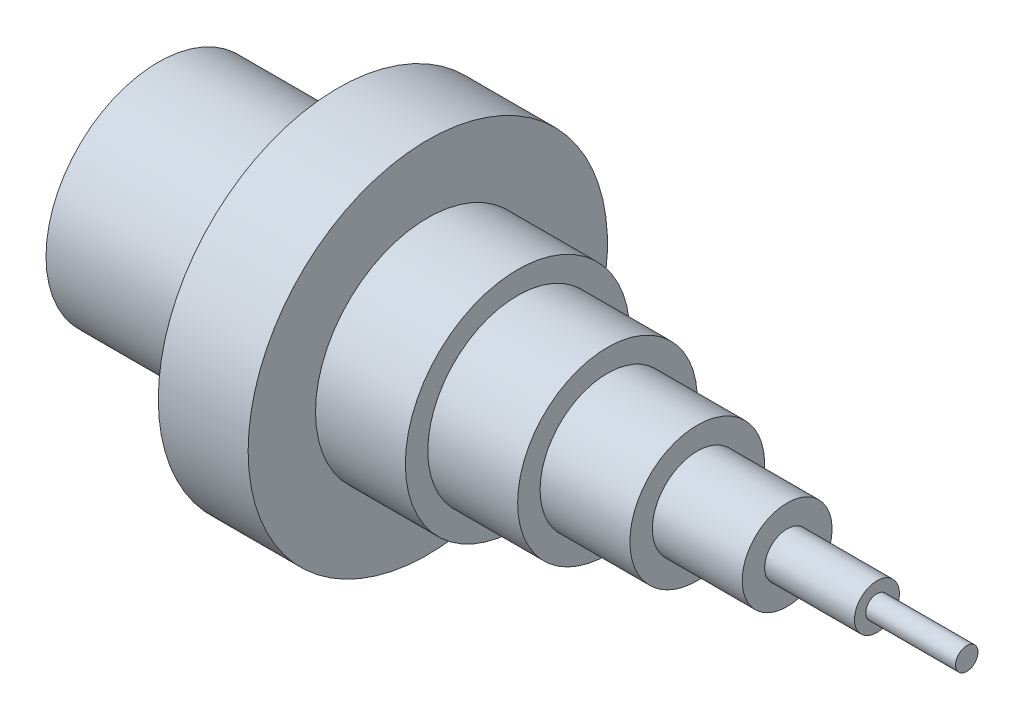
ISO-10303-21;
HEADER;
FILE_DESCRIPTION(('STEP AP214'),'2;1');
FILE_NAME('part.step','',(''),(''),'','','');
FILE_SCHEMA(('AUTOMOTIVE_DESIGN { 1 0 10303 214 1 1 1 1 }'));
ENDSEC;
DATA;
#1=APPLICATION_CONTEXT('core data for automotive mechanical design processes');
#2=APPLICATION_PROTOCOL_DEFINITION('international standard','automotive_design',2000,#1);
#3=PRODUCT_CONTEXT('',#1,'mechanical');
#4=PRODUCT('Part','Part','',(#3));
#5=PRODUCT_RELATED_PRODUCT_CATEGORY('part','',(#4));
#6=PRODUCT_DEFINITION_FORMATION('','',#4);
#7=PRODUCT_DEFINITION_CONTEXT('part definition',#1,'design');
#8=PRODUCT_DEFINITION('design','',#6,#7);
#9=PRODUCT_DEFINITION_SHAPE('','',#8);
#10=(LENGTH_UNIT() NAMED_UNIT(*) SI_UNIT(.MILLI.,.METRE.));
#11=(NAMED_UNIT(*) PLANE_ANGLE_UNIT() SI_UNIT($,.RADIAN.));
#12=(NAMED_UNIT(*) SI_UNIT($,.STERADIAN.) SOLID_ANGLE_UNIT());
#13=UNCERTAINTY_MEASURE_WITH_UNIT(LENGTH_MEASURE(1.E-05),#10,'distance_accuracy_value','');
#14=(GEOMETRIC_REPRESENTATION_CONTEXT(3) GLOBAL_UNCERTAINTY_ASSIGNED_CONTEXT((#13)) GLOBAL_UNIT_ASSIGNED_CONTEXT((#10,
#11,#12)) REPRESENTATION_CONTEXT('',''));
#15=CARTESIAN_POINT('',(0.,0.,0.));
#16=DIRECTION('',(0.,0.,1.));
#17=DIRECTION('',(1.,0.,0.));
#18=AXIS2_PLACEMENT_3D('',#15,#16,#17);
#19=CARTESIAN_POINT('',(-40.,0.,0.));
#20=DIRECTION('',(1.,0.,0.));
#21=DIRECTION('',(0.,0.,-1.));
#22=AXIS2_PLACEMENT_3D('',#19,#20,#21);
#23=PLANE('',#22);
#24=CARTESIAN_POINT('',(-40.,0.,0.));
#25=DIRECTION('',(-1.,0.,0.));
#26=DIRECTION('',(0.,0.,1.));
#27=AXIS2_PLACEMENT_3D('',#24,#25,#26);
#28=CIRCLE('',#27,20.);
#29=CARTESIAN_POINT('',(-40.,0.,20.));
#30=VERTEX_POINT('',#29);
#31=EDGE_CURVE('E92',#30,#30,#28,.T.);
#32=ORIENTED_EDGE('',*,*,#31,.F.);
#33=EDGE_LOOP('',(#32));
#34=FACE_BOUND('',#33,.T.);
#35=CARTESIAN_POINT('',(-40.,0.,0.));
#36=DIRECTION('',(-1.,0.,0.));
#37=DIRECTION('',(0.,0.,1.));
#38=AXIS2_PLACEMENT_3D('',#35,#36,#37);
#39=CIRCLE('',#38,25.);
#40=CARTESIAN_POINT('',(-40.,0.,25.));
#41=VERTEX_POINT('',#40);
#42=EDGE_CURVE('E10',#41,#41,#39,.T.);
#43=ORIENTED_EDGE('',*,*,#42,.T.);
#44=EDGE_LOOP('',(#43));
#45=FACE_BOUND('',#44,.T.);
#46=ADVANCED_FACE('F39',(#34,#45),#23,.F.);
#47=CARTESIAN_POINT('',(-63.8506512875603,0.,0.));
#48=DIRECTION('',(-1.,0.,0.));
#49=DIRECTION('',(0.,0.,1.));
#50=AXIS2_PLACEMENT_3D('',#47,#48,#49);
#51=CYLINDRICAL_SURFACE('',#50,25.);
#52=ORIENTED_EDGE('',*,*,#42,.F.);
#53=EDGE_LOOP('',(#52));
#54=FACE_BOUND('',#53,.T.);
#55=CARTESIAN_POINT('',(0.,0.,0.));
#56=DIRECTION('',(-1.,0.,0.));
#57=DIRECTION('',(0.,0.,1.));
#58=AXIS2_PLACEMENT_3D('',#55,#56,#57);
#59=CIRCLE('',#58,25.);
#60=CARTESIAN_POINT('',(0.,0.,25.));
#61=VERTEX_POINT('',#60);
#62=EDGE_CURVE('E44',#61,#61,#59,.T.);
#63=ORIENTED_EDGE('',*,*,#62,.T.);
#64=EDGE_LOOP('',(#63));
#65=FACE_BOUND('',#64,.T.);
#66=ADVANCED_FACE('F112',(#54,#65),#51,.T.);
#67=CARTESIAN_POINT('',(0.,25.,0.));
#68=DIRECTION('',(1.,0.,0.));
#69=DIRECTION('',(0.,0.,-1.));
#70=AXIS2_PLACEMENT_3D('',#67,#68,#69);
#71=PLANE('',#70);
#72=ORIENTED_EDGE('',*,*,#62,.F.);
#73=EDGE_LOOP('',(#72));
#74=FACE_BOUND('',#73,.T.);
#75=CARTESIAN_POINT('',(0.,0.,0.));
#76=DIRECTION('',(-1.,0.,0.));
#77=DIRECTION('',(0.,0.,1.));
#78=AXIS2_PLACEMENT_3D('',#75,#76,#77);
#79=CIRCLE('',#78,40.);
#80=CARTESIAN_POINT('',(0.,0.,40.));
#81=VERTEX_POINT('',#80);
#82=EDGE_CURVE('E47',#81,#81,#79,.T.);
#83=ORIENTED_EDGE('',*,*,#82,.T.);
#84=EDGE_LOOP('',(#83));
#85=FACE_BOUND('',#84,.T.);
#86=ADVANCED_FACE('F116',(#74,#85),#71,.F.);
#87=CARTESIAN_POINT('',(-63.8506512875603,0.,0.));
#88=DIRECTION('',(-1.,0.,0.));
#89=DIRECTION('',(0.,0.,1.));
#90=AXIS2_PLACEMENT_3D('',#87,#88,#89);
#91=CYLINDRICAL_SURFACE('',#90,40.);
#92=ORIENTED_EDGE('',*,*,#82,.F.);
#93=EDGE_LOOP('',(#92));
#94=FACE_BOUND('',#93,.T.);
#95=CARTESIAN_POINT('',(20.,0.,0.));
#96=DIRECTION('',(-1.,0.,0.));
#97=DIRECTION('',(0.,0.,1.));
#98=AXIS2_PLACEMENT_3D('',#95,#96,#97);
#99=CIRCLE('',#98,40.);
#100=CARTESIAN_POINT('',(20.,0.,40.));
#101=VERTEX_POINT('',#100);
#102=EDGE_CURVE('E52',#101,#101,#99,.T.);
#103=ORIENTED_EDGE('',*,*,#102,.T.);
#104=EDGE_LOOP('',(#103));
#105=FACE_BOUND('',#104,.T.);
#106=ADVANCED_FACE('F122',(#94,#105),#91,.T.);
#107=CARTESIAN_POINT('',(20.,40.,0.));
#108=DIRECTION('',(-1.,0.,0.));
#109=DIRECTION('',(0.,0.,1.));
#110=AXIS2_PLACEMENT_3D('',#107,#108,#109);
#111=PLANE('',#110);
#112=ORIENTED_EDGE('',*,*,#102,.F.);
#113=EDGE_LOOP('',(#112));
#114=FACE_BOUND('',#113,.T.);
#115=CARTESIAN_POINT('',(20.,0.,0.));
#116=DIRECTION('',(-1.,0.,0.));
#117=DIRECTION('',(0.,0.,1.));
#118=AXIS2_PLACEMENT_3D('',#115,#116,#117);
#119=CIRCLE('',#118,25.);
#120=CARTESIAN_POINT('',(20.,0.,25.));
#121=VERTEX_POINT('',#120);
#122=EDGE_CURVE('E59',#121,#121,#119,.T.);
#123=ORIENTED_EDGE('',*,*,#122,.T.);
#124=EDGE_LOOP('',(#123));
#125=FACE_BOUND('',#124,.T.);
#126=ADVANCED_FACE('F130',(#114,#125),#111,.F.);
#127=CARTESIAN_POINT('',(-63.8506512875603,0.,0.));
#128=DIRECTION('',(-1.,0.,0.));
#129=DIRECTION('',(0.,0.,1.));
#130=AXIS2_PLACEMENT_3D('',#127,#128,#129);
#131=CYLINDRICAL_SURFACE('',#130,25.);
#132=ORIENTED_EDGE('',*,*,#122,.F.);
#133=EDGE_LOOP('',(#132));
#134=FACE_BOUND('',#133,.T.);
#135=CARTESIAN_POINT('',(40.,0.,0.));
#136=DIRECTION('',(-1.,0.,0.));
#137=DIRECTION('',(0.,0.,1.));
#138=AXIS2_PLACEMENT_3D('',#135,#136,#137);
#139=CIRCLE('',#138,25.);
#140=CARTESIAN_POINT('',(40.,0.,25.));
#141=VERTEX_POINT('',#140);
#142=EDGE_CURVE('E61',#141,#141,#139,.T.);
#143=ORIENTED_EDGE('',*,*,#142,.T.);
#144=EDGE_LOOP('',(#143));
#145=FACE_BOUND('',#144,.T.);
#146=ADVANCED_FACE('F131',(#134,#145),#131,.T.);
#147=CARTESIAN_POINT('',(40.,25.,0.));
#148=DIRECTION('',(-1.,0.,0.));
#149=DIRECTION('',(0.,0.,1.));
#150=AXIS2_PLACEMENT_3D('',#147,#148,#149);
#151=PLANE('',#150);
#152=ORIENTED_EDGE('',*,*,#142,.F.);
#153=EDGE_LOOP('',(#152));
#154=FACE_BOUND('',#153,.T.);
#155=CARTESIAN_POINT('',(40.,0.,0.));
#156=DIRECTION('',(-1.,0.,0.));
#157=DIRECTION('',(0.,0.,1.));
#158=AXIS2_PLACEMENT_3D('',#155,#156,#157);
#159=CIRCLE('',#158,20.);
#160=CARTESIAN_POINT('',(40.,0.,20.));
#161=VERTEX_POINT('',#160);
#162=EDGE_CURVE('E63',#161,#161,#159,.T.);
#163=ORIENTED_EDGE('',*,*,#162,.T.);
#164=EDGE_LOOP('',(#163));
#165=FACE_BOUND('',#164,.T.);
#166=ADVANCED_FACE('F134',(#154,#165),#151,.F.);
#167=CARTESIAN_POINT('',(-63.8506512875603,0.,0.));
#168=DIRECTION('',(-1.,0.,0.));
#169=DIRECTION('',(0.,0.,1.));
#170=AXIS2_PLACEMENT_3D('',#167,#168,#169);
#171=CYLINDRICAL_SURFACE('',#170,20.);
#172=ORIENTED_EDGE('',*,*,#162,.F.);
#173=EDGE_LOOP('',(#172));
#174=FACE_BOUND('',#173,.T.);
#175=CARTESIAN_POINT('',(60.,0.,0.));
#176=DIRECTION('',(-1.,0.,0.));
#177=DIRECTION('',(0.,0.,1.));
#178=AXIS2_PLACEMENT_3D('',#175,#176,#177);
#179=CIRCLE('',#178,20.);
#180=CARTESIAN_POINT('',(60.,0.,20.));
#181=VERTEX_POINT('',#180);
#182=EDGE_CURVE('E70',#181,#181,#179,.T.);
#183=ORIENTED_EDGE('',*,*,#182,.T.);
#184=EDGE_LOOP('',(#183));
#185=FACE_BOUND('',#184,.T.);
#186=ADVANCED_FACE('F136',(#174,#185),#171,.T.);
#187=CARTESIAN_POINT('',(60.,20.,0.));
#188=DIRECTION('',(-1.,0.,0.));
#189=DIRECTION('',(0.,0.,1.));
#190=AXIS2_PLACEMENT_3D('',#187,#188,#189);
#191=PLANE('',#190);
#192=ORIENTED_EDGE('',*,*,#182,.F.);
#193=EDGE_LOOP('',(#192));
#194=FACE_BOUND('',#193,.T.);
#195=CARTESIAN_POINT('',(60.,0.,0.));
#196=DIRECTION('',(-1.,0.,0.));
#197=DIRECTION('',(0.,0.,1.));
#198=AXIS2_PLACEMENT_3D('',#195,#196,#197);
#199=CIRCLE('',#198,15.);
#200=CARTESIAN_POINT('',(60.,0.,15.));
#201=VERTEX_POINT('',#200);
#202=EDGE_CURVE('E68',#201,#201,#199,.T.);
#203=ORIENTED_EDGE('',*,*,#202,.T.);
#204=EDGE_LOOP('',(#203));
#205=FACE_BOUND('',#204,.T.);
#206=ADVANCED_FACE('F141',(#194,#205),#191,.F.);
#207=CARTESIAN_POINT('',(-63.8506512875603,0.,0.));
#208=DIRECTION('',(-1.,0.,0.));
#209=DIRECTION('',(0.,0.,1.));
#210=AXIS2_PLACEMENT_3D('',#207,#208,#209);
#211=CYLINDRICAL_SURFACE('',#210,15.);
#212=ORIENTED_EDGE('',*,*,#202,.F.);
#213=EDGE_LOOP('',(#212));
#214=FACE_BOUND('',#213,.T.);
#215=CARTESIAN_POINT('',(80.,0.,0.));
#216=DIRECTION('',(-1.,0.,0.));
#217=DIRECTION('',(0.,0.,1.));
#218=AXIS2_PLACEMENT_3D('',#215,#216,#217);
#219=CIRCLE('',#218,15.);
#220=CARTESIAN_POINT('',(80.,0.,15.));
#221=VERTEX_POINT('',#220);
#222=EDGE_CURVE('E71',#221,#221,#219,.T.);
#223=ORIENTED_EDGE('',*,*,#222,.T.);
#224=EDGE_LOOP('',(#223));
#225=FACE_BOUND('',#224,.T.);
#226=ADVANCED_FACE('F150',(#214,#225),#211,.T.);
#227=CARTESIAN_POINT('',(80.,15.,0.));
#228=DIRECTION('',(-1.,0.,0.));
#229=DIRECTION('',(0.,0.,1.));
#230=AXIS2_PLACEMENT_3D('',#227,#228,#229);
#231=PLANE('',#230);
#232=ORIENTED_EDGE('',*,*,#222,.F.);
#233=EDGE_LOOP('',(#232));
#234=FACE_BOUND('',#233,.T.);
#235=CARTESIAN_POINT('',(80.,0.,0.));
#236=DIRECTION('',(-1.,0.,0.));
#237=DIRECTION('',(0.,0.,1.));
#238=AXIS2_PLACEMENT_3D('',#235,#236,#237);
#239=CIRCLE('',#238,10.);
#240=CARTESIAN_POINT('',(80.,0.,10.));
#241=VERTEX_POINT('',#240);
#242=EDGE_CURVE('E76',#241,#241,#239,.T.);
#243=ORIENTED_EDGE('',*,*,#242,.T.);
#244=EDGE_LOOP('',(#243));
#245=FACE_BOUND('',#244,.T.);
#246=ADVANCED_FACE('F151',(#234,#245),#231,.F.);
#247=CARTESIAN_POINT('',(-63.8506512875603,0.,0.));
#248=DIRECTION('',(-1.,0.,0.));
#249=DIRECTION('',(0.,0.,1.));
#250=AXIS2_PLACEMENT_3D('',#247,#248,#249);
#251=CYLINDRICAL_SURFACE('',#250,10.);
#252=ORIENTED_EDGE('',*,*,#242,.F.);
#253=EDGE_LOOP('',(#252));
#254=FACE_BOUND('',#253,.T.);
#255=CARTESIAN_POINT('',(100.,0.,0.));
#256=DIRECTION('',(-1.,0.,0.));
#257=DIRECTION('',(0.,0.,1.));
#258=AXIS2_PLACEMENT_3D('',#255,#256,#257);
#259=CIRCLE('',#258,10.);
#260=CARTESIAN_POINT('',(100.,0.,10.));
#261=VERTEX_POINT('',#260);
#262=EDGE_CURVE('E78',#261,#261,#259,.T.);
#263=ORIENTED_EDGE('',*,*,#262,.T.);
#264=EDGE_LOOP('',(#263));
#265=FACE_BOUND('',#264,.T.);
#266=ADVANCED_FACE('F154',(#254,#265),#251,.T.);
#267=CARTESIAN_POINT('',(100.,10.,0.));
#268=DIRECTION('',(-1.,0.,0.));
#269=DIRECTION('',(0.,0.,1.));
#270=AXIS2_PLACEMENT_3D('',#267,#268,#269);
#271=PLANE('',#270);
#272=ORIENTED_EDGE('',*,*,#262,.F.);
#273=EDGE_LOOP('',(#272));
#274=FACE_BOUND('',#273,.T.);
#275=CARTESIAN_POINT('',(100.,0.,0.));
#276=DIRECTION('',(-1.,0.,0.));
#277=DIRECTION('',(0.,0.,1.));
#278=AXIS2_PLACEMENT_3D('',#275,#276,#277);
#279=CIRCLE('',#278,5.);
#280=CARTESIAN_POINT('',(100.,0.,5.));
#281=VERTEX_POINT('',#280);
#282=EDGE_CURVE('E85',#281,#281,#279,.T.);
#283=ORIENTED_EDGE('',*,*,#282,.T.);
#284=EDGE_LOOP('',(#283));
#285=FACE_BOUND('',#284,.T.);
#286=ADVANCED_FACE('F157',(#274,#285),#271,.F.);
#287=CARTESIAN_POINT('',(-63.8506512875603,0.,0.));
#288=DIRECTION('',(-1.,0.,0.));
#289=DIRECTION('',(0.,0.,1.));
#290=AXIS2_PLACEMENT_3D('',#287,#288,#289);
#291=CYLINDRICAL_SURFACE('',#290,5.);
#292=ORIENTED_EDGE('',*,*,#282,.F.);
#293=EDGE_LOOP('',(#292));
#294=FACE_BOUND('',#293,.T.);
#295=CARTESIAN_POINT('',(120.,0.,0.));
#296=DIRECTION('',(-1.,0.,0.));
#297=DIRECTION('',(0.,0.,1.));
#298=AXIS2_PLACEMENT_3D('',#295,#296,#297);
#299=CIRCLE('',#298,5.);
#300=CARTESIAN_POINT('',(120.,0.,5.));
#301=VERTEX_POINT('',#300);
#302=EDGE_CURVE('E83',#301,#301,#299,.T.);
#303=ORIENTED_EDGE('',*,*,#302,.T.);
#304=EDGE_LOOP('',(#303));
#305=FACE_BOUND('',#304,.T.);
#306=ADVANCED_FACE('F162',(#294,#305),#291,.T.);
#307=CARTESIAN_POINT('',(120.,5.,0.));
#308=DIRECTION('',(-1.,0.,0.));
#309=DIRECTION('',(0.,0.,1.));
#310=AXIS2_PLACEMENT_3D('',#307,#308,#309);
#311=PLANE('',#310);
#312=ORIENTED_EDGE('',*,*,#302,.F.);
#313=EDGE_LOOP('',(#312));
#314=FACE_BOUND('',#313,.T.);
#315=CARTESIAN_POINT('',(120.,0.,0.));
#316=DIRECTION('',(-1.,0.,0.));
#317=DIRECTION('',(0.,0.,1.));
#318=AXIS2_PLACEMENT_3D('',#315,#316,#317);
#319=CIRCLE('',#318,2.5);
#320=CARTESIAN_POINT('',(120.,0.,2.5));
#321=VERTEX_POINT('',#320);
#322=EDGE_CURVE('E86',#321,#321,#319,.T.);
#323=ORIENTED_EDGE('',*,*,#322,.T.);
#324=EDGE_LOOP('',(#323));
#325=FACE_BOUND('',#324,.T.);
#326=ADVANCED_FACE('F170',(#314,#325),#311,.F.);
#327=CARTESIAN_POINT('',(-63.8506512875603,0.,0.));
#328=DIRECTION('',(-1.,0.,0.));
#329=DIRECTION('',(0.,0.,1.));
#330=AXIS2_PLACEMENT_3D('',#327,#328,#329);
#331=CYLINDRICAL_SURFACE('',#330,2.5);
#332=ORIENTED_EDGE('',*,*,#322,.F.);
#333=EDGE_LOOP('',(#332));
#334=FACE_BOUND('',#333,.T.);
#335=CARTESIAN_POINT('',(140.,0.,0.));
#336=DIRECTION('',(-1.,0.,0.));
#337=DIRECTION('',(0.,0.,1.));
#338=AXIS2_PLACEMENT_3D('',#335,#336,#337);
#339=CIRCLE('',#338,2.5);
#340=CARTESIAN_POINT('',(140.,0.,2.5));
#341=VERTEX_POINT('',#340);
#342=EDGE_CURVE('E93',#341,#341,#339,.T.);
#343=ORIENTED_EDGE('',*,*,#342,.T.);
#344=EDGE_LOOP('',(#343));
#345=FACE_BOUND('',#344,.T.);
#346=ADVANCED_FACE('F171',(#334,#345),#331,.T.);
#347=CARTESIAN_POINT('',(140.,2.5,0.));
#348=DIRECTION('',(-1.,0.,0.));
#349=DIRECTION('',(0.,0.,1.));
#350=AXIS2_PLACEMENT_3D('',#347,#348,#349);
#351=PLANE('',#350);
#352=ORIENTED_EDGE('',*,*,#342,.F.);
#353=EDGE_LOOP('',(#352));
#354=FACE_BOUND('',#353,.T.);
#355=ADVANCED_FACE('F106',(#354),#351,.F.);
#356=CARTESIAN_POINT('',(0.,0.,0.));
#357=DIRECTION('',(-1.,0.,0.));
#358=DIRECTION('',(0.,0.,1.));
#359=AXIS2_PLACEMENT_3D('',#356,#357,#358);
#360=CYLINDRICAL_SURFACE('',#359,20.);
#361=CARTESIAN_POINT('',(0.,0.,0.));
#362=DIRECTION('',(-1.,0.,0.));
#363=DIRECTION('',(0.,0.,1.));
#364=AXIS2_PLACEMENT_3D('',#361,#362,#363);
#365=CIRCLE('',#364,20.);
#366=CARTESIAN_POINT('',(0.,0.,20.));
#367=VERTEX_POINT('',#366);
#368=EDGE_CURVE('E94',#367,#367,#365,.T.);
#369=ORIENTED_EDGE('',*,*,#368,.F.);
#370=EDGE_LOOP('',(#369));
#371=FACE_BOUND('',#370,.T.);
#372=ORIENTED_EDGE('',*,*,#31,.T.);
#373=EDGE_LOOP('',(#372));
#374=FACE_BOUND('',#373,.T.);
#375=ADVANCED_FACE('F103',(#371,#374),#360,.F.);
#376=CARTESIAN_POINT('',(0.,0.,0.));
#377=DIRECTION('',(-1.,0.,0.));
#378=DIRECTION('',(0.,0.,1.));
#379=AXIS2_PLACEMENT_3D('',#376,#377,#378);
#380=PLANE('',#379);
#381=ORIENTED_EDGE('',*,*,#368,.T.);
#382=EDGE_LOOP('',(#381));
#383=FACE_BOUND('',#382,.T.);
#384=ADVANCED_FACE('F101',(#383),#380,.T.);
#385=CLOSED_SHELL('',(#46,#66,#86,#106,#126,#146,#166,#186,#206,#226,#246,#266,#286,#306,#326,
#346,#355,#375,#384));
#386=MANIFOLD_SOLID_BREP('B2',#385);
#387=ADVANCED_BREP_SHAPE_REPRESENTATION('',(#18,#386),#14);
#388=SHAPE_DEFINITION_REPRESENTATION(#9,#387);
ENDSEC;
END-ISO-10303-21;
